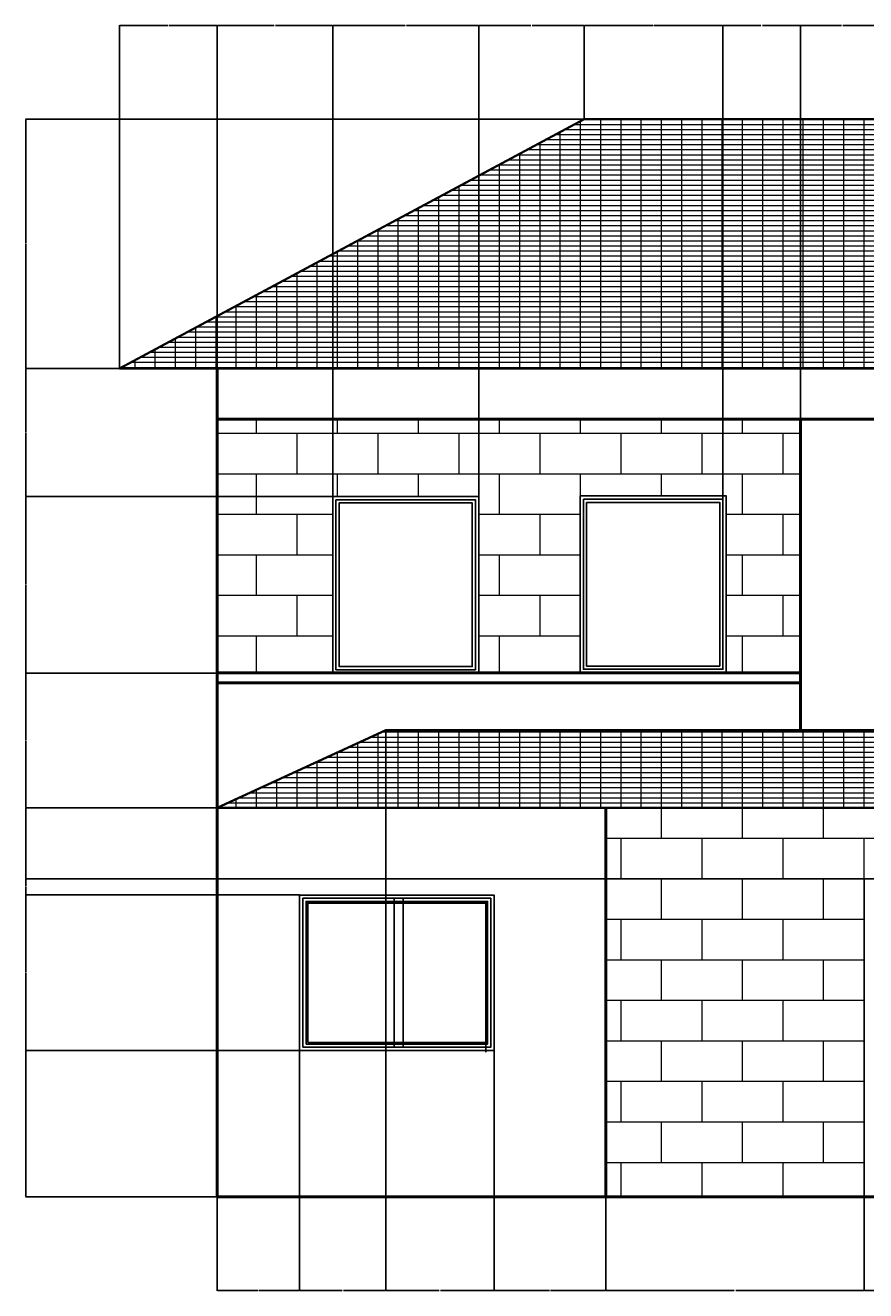
# Model space of a CAD drawing. Units: inches. Extents: x 357 to 1610, y 271 to 1052.
# Tile 1 of 2: x 357 to 876, y 271 to 1052. Entities that reach past the tile are written whole.
import ezdxf

# ---------------------------------------------------------------- set-up
doc = ezdxf.new("R2010")
doc.units = ezdxf.units.IN
doc.header["$MEASUREMENT"] = 0
for name, color, linetype, lineweight in [('A-ANNO-DIMS', 2, 'Continuous', 18), ('A-DOOR', 40, 'Continuous', 25), ('A-GLAZ', 4, 'Continuous', 25), ('A-ROOF', 7, 'Continuous', 35), ('A-ROOF-PATT', 8, 'Continuous', 13), ('A-WALL', 7, 'Continuous', 50), ('A-WALL-PATT', 8, 'Continuous', 18)]:
    doc.layers.add(name, color=color, linetype=linetype, lineweight=lineweight)
doc.styles.get("Standard").update_dxf_attribs({"font": 'arial.ttf'})
doc.dimstyles.get("Standard").update_dxf_attribs({"dimtxt": 0.18, "dimasz": 0.18, "dimexe": 0.18, "dimexo": 0.0625, "dimgap": 0.09, "dimtad": 0, "dimtih": 1, "dimtoh": 1, "dimdec": 4, "dimzin": 0, "dimdsep": 46, "dimtxsty": 'Standard', "dimcen": 0.09, "dimadec": 0, "dimazin": 0, "dimtfac": 1, "dimtdec": 4, "dimtofl": 0, "dimtmove": 0, "dimatfit": 3, "dimfxl": 1, "dimtolj": 1, "dimtzin": 0, "dimarcsym": 0})

# ---------------------------------------------------------------- blocks, each defined once
blk = doc.blocks.new('WIN-900x1090')
for points in [[(0, 108.96), (90.12, 108.96), (90.12, 0), (0, 0)], [(2, 106.96), (88.12, 106.96), (88.12, 2), (2, 2)], [(4, 104.96), (86.12, 104.96), (86.12, 4), (4, 4)]]:
    blk.add_lwpolyline(points, close=True)
blk = doc.blocks.new('*D4')
at = {"layer": 'A-ANNO-DIMS', "color": 0, "lineweight": -2, "transparency": 16777216}
for p, q in [((415.45, 839.95), (415.45, 1051.75)), ((415.63, 1051.57), (445.17, 1051.57)), ((475.49, 1051.57), (445.95, 1051.57)), ((475.67, 839.95), (475.67, 1051.75))]:
    blk.add_line(p, q, dxfattribs=at)
at = {"layer": 'A-ANNO-DIMS', "color": 0, "transparency": 16777216}
for points in [[(415.63, 1051.6), (415.63, 1051.54), (415.45, 1051.57)], [(475.49, 1051.6), (475.49, 1051.54), (475.67, 1051.57)]]:
    blk.add_solid(points, dxfattribs=at)
at = {"layer": 'Defpoints', "color": 0, "transparency": 16777216}
for p in [(475.67, 1051.57), (415.45, 839.89), (475.67, 839.89)]:
    blk.add_point(p, dxfattribs=at)
at = {"layer": 'A-ANNO-DIMS', "color": 0, "transparency": 16777216, "insert": (445.56, 1051.57), "char_height": 0.18, "attachment_point": 5}
blk.add_mtext('\\A1;60.22', dxfattribs=at)
blk = doc.blocks.new('*D5')
at = {"layer": 'A-ANNO-DIMS', "color": 0, "lineweight": -2, "transparency": 16777216}
for p, q in [((475.67, 839.95), (475.67, 1051.75)), ((475.85, 1051.57), (510.96, 1051.57)), ((546.85, 1051.57), (511.74, 1051.57)), ((547.03, 761.02), (547.03, 1051.75))]:
    blk.add_line(p, q, dxfattribs=at)
at = {"layer": 'A-ANNO-DIMS', "color": 0, "transparency": 16777216}
for points in [[(475.85, 1051.6), (475.85, 1051.54), (475.67, 1051.57)], [(546.85, 1051.6), (546.85, 1051.54), (547.03, 1051.57)]]:
    blk.add_solid(points, dxfattribs=at)
at = {"layer": 'Defpoints', "color": 0, "transparency": 16777216}
for p in [(547.03, 1051.57), (475.67, 839.89), (547.03, 760.96)]:
    blk.add_point(p, dxfattribs=at)
at = {"layer": 'A-ANNO-DIMS', "color": 0, "transparency": 16777216, "insert": (511.35, 1051.57), "char_height": 0.18, "attachment_point": 5}
blk.add_mtext('\\A1;71.36', dxfattribs=at)
blk = doc.blocks.new('*D6')
at = {"layer": 'A-ANNO-DIMS', "color": 0, "lineweight": -2, "transparency": 16777216}
for p, q in [((547.03, 761.02), (547.03, 1051.75)), ((547.21, 1051.57), (591.7, 1051.57)), ((636.97, 1051.57), (592.49, 1051.57)), ((637.15, 761.02), (637.15, 1051.75))]:
    blk.add_line(p, q, dxfattribs=at)
at = {"layer": 'A-ANNO-DIMS', "color": 0, "transparency": 16777216}
for points in [[(547.21, 1051.6), (547.21, 1051.54), (547.03, 1051.57)], [(636.97, 1051.6), (636.97, 1051.54), (637.15, 1051.57)]]:
    blk.add_solid(points, dxfattribs=at)
at = {"layer": 'Defpoints', "color": 0, "transparency": 16777216}
for p in [(637.15, 1051.57), (547.03, 760.96), (637.15, 760.96)]:
    blk.add_point(p, dxfattribs=at)
at = {"layer": 'A-ANNO-DIMS', "color": 0, "transparency": 16777216, "insert": (592.09, 1051.57), "char_height": 0.18, "attachment_point": 5}
blk.add_mtext('\\A1;90.12', dxfattribs=at)
blk = doc.blocks.new('*D7')
at = {"layer": 'A-ANNO-DIMS', "color": 0, "lineweight": -2, "transparency": 16777216}
for p, q in [((637.15, 761.02), (637.15, 1051.75)), ((637.33, 1051.57), (669.33, 1051.57)), ((702.11, 1051.57), (670.12, 1051.57)), ((702.29, 993.83), (702.29, 1051.75))]:
    blk.add_line(p, q, dxfattribs=at)
at = {"layer": 'A-ANNO-DIMS', "color": 0, "transparency": 16777216}
for points in [[(637.33, 1051.6), (637.33, 1051.54), (637.15, 1051.57)], [(702.11, 1051.6), (702.11, 1051.54), (702.29, 1051.57)]]:
    blk.add_solid(points, dxfattribs=at)
at = {"layer": 'Defpoints', "color": 0, "transparency": 16777216}
for p in [(702.29, 1051.57), (702.29, 993.77), (637.15, 760.96)]:
    blk.add_point(p, dxfattribs=at)
at = {"layer": 'A-ANNO-DIMS', "color": 0, "transparency": 16777216, "insert": (669.72, 1051.57), "char_height": 0.18, "attachment_point": 5}
blk.add_mtext('\\A1;65.14', dxfattribs=at)
blk = doc.blocks.new('*D8')
at = {"layer": 'A-ANNO-DIMS', "color": 0, "lineweight": -2, "transparency": 16777216}
for p, q in [((702.29, 993.83), (702.29, 1051.75)), ((702.47, 1051.57), (744.76, 1051.57)), ((787.7, 1051.57), (745.41, 1051.57)), ((787.88, 759.31), (787.88, 1051.75))]:
    blk.add_line(p, q, dxfattribs=at)
at = {"layer": 'A-ANNO-DIMS', "color": 0, "transparency": 16777216}
for points in [[(702.47, 1051.6), (702.47, 1051.54), (702.29, 1051.57)], [(787.7, 1051.6), (787.7, 1051.54), (787.88, 1051.57)]]:
    blk.add_solid(points, dxfattribs=at)
at = {"layer": 'Defpoints', "color": 0, "transparency": 16777216}
for p in [(787.88, 1051.57), (702.29, 993.77), (787.88, 759.25)]:
    blk.add_point(p, dxfattribs=at)
at = {"layer": 'A-ANNO-DIMS', "color": 0, "transparency": 16777216, "insert": (745.09, 1051.57), "char_height": 0.18, "attachment_point": 5}
blk.add_mtext('\\A1;85.6', dxfattribs=at)
blk = doc.blocks.new('*D9')
at = {"layer": 'A-ANNO-DIMS', "color": 0, "lineweight": -2, "transparency": 16777216}
for p, q in [((787.88, 759.31), (787.88, 1051.75)), ((788.06, 1051.57), (811.31, 1051.57)), ((835.49, 1051.57), (812.25, 1051.57)), ((835.67, 808.83), (835.67, 1051.75))]:
    blk.add_line(p, q, dxfattribs=at)
at = {"layer": 'A-ANNO-DIMS', "color": 0, "transparency": 16777216}
for points in [[(788.06, 1051.6), (788.06, 1051.54), (787.88, 1051.57)], [(835.49, 1051.6), (835.49, 1051.54), (835.67, 1051.57)]]:
    blk.add_solid(points, dxfattribs=at)
at = {"layer": 'Defpoints', "color": 0, "transparency": 16777216}
for p in [(835.67, 1051.57), (835.67, 808.77), (787.88, 759.25)]:
    blk.add_point(p, dxfattribs=at)
at = {"layer": 'A-ANNO-DIMS', "color": 0, "transparency": 16777216, "insert": (811.78, 1051.57), "char_height": 0.18, "attachment_point": 5}
blk.add_mtext('\\A1;47.785', dxfattribs=at)
blk = doc.blocks.new('*D10')
at = {"layer": 'A-ANNO-DIMS', "color": 0, "lineweight": -2, "transparency": 16777216}
for p, q in [((835.67, 808.83), (835.67, 1051.75)), ((835.85, 1051.57), (861.05, 1051.57)), ((887.04, 1051.57), (861.84, 1051.57)), ((887.22, 769.8), (887.22, 1051.75))]:
    blk.add_line(p, q, dxfattribs=at)
at = {"layer": 'A-ANNO-DIMS', "color": 0, "transparency": 16777216}
for points in [[(835.85, 1051.6), (835.85, 1051.54), (835.67, 1051.57)], [(887.04, 1051.6), (887.04, 1051.54), (887.22, 1051.57)]]:
    blk.add_solid(points, dxfattribs=at)
at = {"layer": 'Defpoints', "color": 0, "transparency": 16777216}
for p in [(887.22, 1051.57), (835.67, 808.77), (887.22, 769.73)]:
    blk.add_point(p, dxfattribs=at)
at = {"layer": 'A-ANNO-DIMS', "color": 0, "transparency": 16777216, "insert": (861.44, 1051.57), "char_height": 0.18, "attachment_point": 5}
blk.add_mtext('\\A1;51.55', dxfattribs=at)
blk = doc.blocks.new('*D22')
at = {"layer": 'A-ANNO-DIMS', "color": 0, "lineweight": -2, "transparency": 16777216}
for p, q in [((526.59, 418.93), (526.59, 270.79)), ((475.67, 328.7), (475.67, 270.79)), ((475.85, 270.97), (500.74, 270.97)), ((526.41, 270.97), (501.52, 270.97))]:
    blk.add_line(p, q, dxfattribs=at)
at = {"layer": 'A-ANNO-DIMS', "color": 0, "transparency": 16777216}
for points in [[(475.85, 271), (475.85, 270.94), (475.67, 270.97)], [(526.41, 271), (526.41, 270.94), (526.59, 270.97)]]:
    blk.add_solid(points, dxfattribs=at)
at = {"layer": 'Defpoints', "color": 0, "transparency": 16777216}
for p in [(526.59, 419), (475.67, 328.77), (526.59, 270.97)]:
    blk.add_point(p, dxfattribs=at)
at = {"layer": 'A-ANNO-DIMS', "color": 0, "transparency": 16777216, "insert": (501.13, 270.97), "char_height": 0.18, "attachment_point": 5}
blk.add_mtext('\\A1;50.92', dxfattribs=at)
blk = doc.blocks.new('*D23')
at = {"layer": 'A-ANNO-DIMS', "color": 0, "lineweight": -2, "transparency": 16777216}
for p, q in [((579.84, 616.7), (579.84, 270.79)), ((526.59, 418.93), (526.59, 270.79)), ((526.77, 270.97), (552.82, 270.97)), ((579.66, 270.97), (553.61, 270.97))]:
    blk.add_line(p, q, dxfattribs=at)
at = {"layer": 'A-ANNO-DIMS', "color": 0, "transparency": 16777216}
for points in [[(526.77, 271), (526.77, 270.94), (526.59, 270.97)], [(579.66, 271), (579.66, 270.94), (579.84, 270.97)]]:
    blk.add_solid(points, dxfattribs=at)
at = {"layer": 'Defpoints', "color": 0, "transparency": 16777216}
for p in [(579.84, 616.77), (526.59, 419), (579.84, 270.97)]:
    blk.add_point(p, dxfattribs=at)
at = {"layer": 'A-ANNO-DIMS', "color": 0, "transparency": 16777216, "insert": (553.22, 270.97), "char_height": 0.18, "attachment_point": 5}
blk.add_mtext('\\A1;53.25', dxfattribs=at)
blk = doc.blocks.new('*D24')
at = {"layer": 'A-ANNO-DIMS', "color": 0, "lineweight": -2, "transparency": 16777216}
for p, q in [((579.84, 616.7), (579.84, 270.79)), ((646.59, 418.93), (646.59, 270.79)), ((580.02, 270.97), (612.82, 270.97)), ((646.41, 270.97), (613.61, 270.97))]:
    blk.add_line(p, q, dxfattribs=at)
at = {"layer": 'A-ANNO-DIMS', "color": 0, "transparency": 16777216}
for points in [[(580.02, 271), (580.02, 270.94), (579.84, 270.97)], [(646.41, 271), (646.41, 270.94), (646.59, 270.97)]]:
    blk.add_solid(points, dxfattribs=at)
at = {"layer": 'Defpoints', "color": 0, "transparency": 16777216}
for p in [(579.84, 616.77), (646.59, 419), (646.59, 270.97)]:
    blk.add_point(p, dxfattribs=at)
at = {"layer": 'A-ANNO-DIMS', "color": 0, "transparency": 16777216, "insert": (613.22, 270.97), "char_height": 0.18, "attachment_point": 5}
blk.add_mtext('\\A1;66.75', dxfattribs=at)
blk = doc.blocks.new('*D25')
at = {"layer": 'A-ANNO-DIMS', "color": 0, "lineweight": -2, "transparency": 16777216}
for p, q in [((646.59, 418.93), (646.59, 270.79)), ((715.67, 328.7), (715.67, 270.79)), ((646.77, 270.97), (680.74, 270.97)), ((715.49, 270.97), (681.53, 270.97))]:
    blk.add_line(p, q, dxfattribs=at)
at = {"layer": 'A-ANNO-DIMS', "color": 0, "transparency": 16777216}
for points in [[(646.77, 271), (646.77, 270.94), (646.59, 270.97)], [(715.49, 271), (715.49, 270.94), (715.67, 270.97)]]:
    blk.add_solid(points, dxfattribs=at)
at = {"layer": 'Defpoints', "color": 0, "transparency": 16777216}
for p in [(646.59, 419), (715.67, 328.77), (715.67, 270.97)]:
    blk.add_point(p, dxfattribs=at)
at = {"layer": 'A-ANNO-DIMS', "color": 0, "transparency": 16777216, "insert": (681.13, 270.97), "char_height": 0.18, "attachment_point": 5}
blk.add_mtext('\\A1;69.08', dxfattribs=at)
blk = doc.blocks.new('*D26')
at = {"layer": 'A-ANNO-DIMS', "color": 0, "lineweight": -2, "transparency": 16777216}
for p, q in [((715.67, 328.7), (715.67, 270.79)), ((875, 328.7), (875, 270.79)), ((715.85, 270.97), (794.88, 270.97)), ((874.82, 270.97), (795.79, 270.97))]:
    blk.add_line(p, q, dxfattribs=at)
at = {"layer": 'A-ANNO-DIMS', "color": 0, "transparency": 16777216}
for points in [[(715.85, 271), (715.85, 270.94), (715.67, 270.97)], [(874.82, 271), (874.82, 270.94), (875, 270.97)]]:
    blk.add_solid(points, dxfattribs=at)
at = {"layer": 'Defpoints', "color": 0, "transparency": 16777216}
for p in [(715.67, 328.77), (875, 328.77), (875, 270.97)]:
    blk.add_point(p, dxfattribs=at)
at = {"layer": 'A-ANNO-DIMS', "color": 0, "transparency": 16777216, "insert": (795.33, 270.97), "char_height": 0.18, "attachment_point": 5}
blk.add_mtext('\\A1;159.33', dxfattribs=at)
blk = doc.blocks.new('*D27')
at = {"layer": 'A-ANNO-DIMS', "color": 0, "lineweight": -2, "transparency": 16777216}
for p, q in [((875, 328.7), (875, 270.79)), ((975, 328.7), (975, 270.79)), ((875.18, 270.97), (924.72, 270.97)), ((974.82, 270.97), (925.28, 270.97))]:
    blk.add_line(p, q, dxfattribs=at)
at = {"layer": 'A-ANNO-DIMS', "color": 0, "transparency": 16777216}
for points in [[(875.18, 271), (875.18, 270.94), (875, 270.97)], [(974.82, 271), (974.82, 270.94), (975, 270.97)]]:
    blk.add_solid(points, dxfattribs=at)
at = {"layer": 'Defpoints', "color": 0, "transparency": 16777216}
for p in [(875, 328.77), (975, 328.77), (975, 270.97)]:
    blk.add_point(p, dxfattribs=at)
at = {"layer": 'A-ANNO-DIMS', "color": 0, "transparency": 16777216, "insert": (925, 270.97), "char_height": 0.18, "attachment_point": 5}
blk.add_mtext('\\A1;100', dxfattribs=at)
blk = doc.blocks.new('*D32')
at = {"layer": 'A-ANNO-DIMS', "color": 0, "lineweight": -2, "transparency": 16777216}
for p, q in [((526.53, 419), (357.47, 419)), ((357.65, 418.82), (357.65, 374.06)), ((357.65, 328.95), (357.65, 373.7)), ((475.61, 328.77), (357.47, 328.77))]:
    blk.add_line(p, q, dxfattribs=at)
at = {"layer": 'A-ANNO-DIMS', "color": 0, "transparency": 16777216}
for points in [[(357.62, 418.82), (357.68, 418.82), (357.65, 419)], [(357.62, 328.95), (357.68, 328.95), (357.65, 328.77)]]:
    blk.add_solid(points, dxfattribs=at)
at = {"layer": 'Defpoints', "color": 0, "transparency": 16777216}
for p in [(357.65, 419), (526.59, 419), (475.67, 328.77)]:
    blk.add_point(p, dxfattribs=at)
at = {"layer": 'A-ANNO-DIMS', "color": 0, "transparency": 16777216, "insert": (357.65, 373.88), "char_height": 0.18, "attachment_point": 5}
blk.add_mtext('\\A1;90.23', dxfattribs=at)
blk = doc.blocks.new('*D33')
at = {"layer": 'A-ANNO-DIMS', "color": 0, "lineweight": -2, "transparency": 16777216}
for p, q in [((526.53, 515), (357.47, 515)), ((357.65, 514.82), (357.65, 467.18)), ((357.65, 419.18), (357.65, 466.81)), ((526.53, 419), (357.47, 419))]:
    blk.add_line(p, q, dxfattribs=at)
at = {"layer": 'A-ANNO-DIMS', "color": 0, "transparency": 16777216}
for points in [[(357.62, 514.82), (357.68, 514.82), (357.65, 515)], [(357.62, 419.18), (357.68, 419.18), (357.65, 419)]]:
    blk.add_solid(points, dxfattribs=at)
at = {"layer": 'Defpoints', "color": 0, "transparency": 16777216}
for p in [(357.65, 515), (526.59, 515), (526.59, 419)]:
    blk.add_point(p, dxfattribs=at)
at = {"layer": 'A-ANNO-DIMS', "color": 0, "transparency": 16777216, "insert": (357.65, 467), "char_height": 0.18, "attachment_point": 5}
blk.add_mtext('\\A1;96', dxfattribs=at)
blk = doc.blocks.new('*D34')
at = {"layer": 'A-ANNO-DIMS', "color": 0, "lineweight": -2, "transparency": 16777216}
for p, q in [((874.94, 525), (357.47, 525)), ((357.65, 524.82), (357.65, 520.18)), ((357.65, 515.18), (357.65, 519.82)), ((526.53, 515), (357.47, 515))]:
    blk.add_line(p, q, dxfattribs=at)
at = {"layer": 'A-ANNO-DIMS', "color": 0, "transparency": 16777216}
for points in [[(357.62, 524.82), (357.68, 524.82), (357.65, 525)], [(357.62, 515.18), (357.68, 515.18), (357.65, 515)]]:
    blk.add_solid(points, dxfattribs=at)
at = {"layer": 'Defpoints', "color": 0, "transparency": 16777216}
for p in [(357.65, 525), (875, 525), (526.59, 515)]:
    blk.add_point(p, dxfattribs=at)
at = {"layer": 'A-ANNO-DIMS', "color": 0, "transparency": 16777216, "insert": (357.65, 520), "char_height": 0.18, "attachment_point": 5}
blk.add_mtext('\\A1;10.004', dxfattribs=at)
blk = doc.blocks.new('*D35')
at = {"layer": 'A-ANNO-DIMS', "color": 0, "lineweight": -2, "transparency": 16777216}
for p, q in [((475.61, 568.77), (357.47, 568.77)), ((357.65, 568.59), (357.65, 547.07)), ((357.65, 525.18), (357.65, 546.7)), ((874.94, 525), (357.47, 525))]:
    blk.add_line(p, q, dxfattribs=at)
at = {"layer": 'A-ANNO-DIMS', "color": 0, "transparency": 16777216}
for points in [[(357.62, 568.59), (357.68, 568.59), (357.65, 568.77)], [(357.62, 525.18), (357.68, 525.18), (357.65, 525)]]:
    blk.add_solid(points, dxfattribs=at)
at = {"layer": 'Defpoints', "color": 0, "transparency": 16777216}
for p in [(357.65, 568.77), (475.67, 568.77), (875, 525)]:
    blk.add_point(p, dxfattribs=at)
at = {"layer": 'A-ANNO-DIMS', "color": 0, "transparency": 16777216, "insert": (357.65, 546.88), "char_height": 0.18, "attachment_point": 5}
blk.add_mtext('\\A1;43.77', dxfattribs=at)
blk = doc.blocks.new('*D36')
at = {"layer": 'A-ANNO-DIMS', "color": 0, "lineweight": -2, "transparency": 16777216}
for p, q in [((546.97, 652), (357.47, 652)), ((357.65, 651.82), (357.65, 610.56)), ((357.65, 568.95), (357.65, 610.2)), ((475.61, 568.77), (357.47, 568.77))]:
    blk.add_line(p, q, dxfattribs=at)
at = {"layer": 'A-ANNO-DIMS', "color": 0, "transparency": 16777216}
for points in [[(357.62, 651.82), (357.68, 651.82), (357.65, 652)], [(357.62, 568.95), (357.68, 568.95), (357.65, 568.77)]]:
    blk.add_solid(points, dxfattribs=at)
at = {"layer": 'Defpoints', "color": 0, "transparency": 16777216}
for p in [(357.65, 652), (547.03, 652), (475.67, 568.77)]:
    blk.add_point(p, dxfattribs=at)
at = {"layer": 'A-ANNO-DIMS', "color": 0, "transparency": 16777216, "insert": (357.65, 610.38), "char_height": 0.18, "attachment_point": 5}
blk.add_mtext('\\A1;83.23', dxfattribs=at)
blk = doc.blocks.new('*D37')
at = {"layer": 'A-ANNO-DIMS', "color": 0, "lineweight": -2, "transparency": 16777216}
for p, q in [((546.97, 760.96), (357.47, 760.96)), ((357.65, 760.78), (357.65, 706.66)), ((357.65, 652.18), (357.65, 706.3)), ((546.97, 652), (357.47, 652))]:
    blk.add_line(p, q, dxfattribs=at)
at = {"layer": 'A-ANNO-DIMS', "color": 0, "transparency": 16777216}
for points in [[(357.62, 760.78), (357.68, 760.78), (357.65, 760.96)], [(357.62, 652.18), (357.68, 652.18), (357.65, 652)]]:
    blk.add_solid(points, dxfattribs=at)
at = {"layer": 'Defpoints', "color": 0, "transparency": 16777216}
for p in [(357.65, 760.96), (547.03, 760.96), (547.03, 652)]:
    blk.add_point(p, dxfattribs=at)
at = {"layer": 'A-ANNO-DIMS', "color": 0, "transparency": 16777216, "insert": (357.65, 706.48), "char_height": 0.18, "attachment_point": 5}
blk.add_mtext('\\A1;108.96', dxfattribs=at)
blk = doc.blocks.new('*D38')
at = {"layer": 'A-ANNO-DIMS', "color": 0, "lineweight": -2, "transparency": 16777216}
for p, q in [((415.39, 839.89), (357.47, 839.89)), ((357.65, 839.71), (357.65, 800.61)), ((357.65, 761.14), (357.65, 800.24)), ((546.97, 760.96), (357.47, 760.96))]:
    blk.add_line(p, q, dxfattribs=at)
at = {"layer": 'A-ANNO-DIMS', "color": 0, "transparency": 16777216}
for points in [[(357.62, 839.71), (357.68, 839.71), (357.65, 839.89)], [(357.62, 761.14), (357.68, 761.14), (357.65, 760.96)]]:
    blk.add_solid(points, dxfattribs=at)
at = {"layer": 'Defpoints', "color": 0, "transparency": 16777216}
for p in [(357.65, 839.89), (415.45, 839.89), (547.03, 760.96)]:
    blk.add_point(p, dxfattribs=at)
at = {"layer": 'A-ANNO-DIMS', "color": 0, "transparency": 16777216, "insert": (357.65, 800.42), "char_height": 0.18, "attachment_point": 5}
blk.add_mtext('\\A1;78.93', dxfattribs=at)
blk = doc.blocks.new('*D39')
at = {"layer": 'A-ANNO-DIMS', "color": 0, "lineweight": -2, "transparency": 16777216}
for p, q in [((702.23, 993.77), (357.47, 993.77)), ((357.65, 993.59), (357.65, 917.01)), ((357.65, 840.07), (357.65, 916.65)), ((415.39, 839.89), (357.47, 839.89))]:
    blk.add_line(p, q, dxfattribs=at)
at = {"layer": 'A-ANNO-DIMS', "color": 0, "transparency": 16777216}
for points in [[(357.62, 993.59), (357.68, 993.59), (357.65, 993.77)], [(357.62, 840.07), (357.68, 840.07), (357.65, 839.89)]]:
    blk.add_solid(points, dxfattribs=at)
at = {"layer": 'Defpoints', "color": 0, "transparency": 16777216}
for p in [(357.65, 993.77), (702.29, 993.77), (415.45, 839.89)]:
    blk.add_point(p, dxfattribs=at)
at = {"layer": 'A-ANNO-DIMS', "color": 0, "transparency": 16777216, "insert": (357.65, 916.83), "char_height": 0.18, "attachment_point": 5}
blk.add_mtext('\\A1;153.88', dxfattribs=at)

msp = doc.modelspace()

# ---------------------------------------------------------------- hatches: boundary and pattern name
at = {"layer": 'A-ROOF-PATT'}
h = msp.add_hatch(dxfattribs=at)
h.set_pattern_fill('GRATE', color=256, scale=100)
h.paths.add_polyline_path([(1006.7419, 993.7706), (702.2918, 993.7706), (415.4488, 839.8897), (475.6698, 839.8897), (1435.5868, 839.8897), (1495.8077, 839.8897), (1350.5849, 901.7507), (1169.5186, 901.7507)])
h = msp.add_hatch(dxfattribs=at)
h.set_pattern_fill('GRATE', color=256, scale=100)
h.paths.add_polyline_path([(1435.6698, 616.7674), (579.8425, 616.7674), (475.6698, 568.7674), (1435.6698, 568.7674), (1551.4751, 568.7674)])
at = {"layer": 'A-WALL-PATT'}
h = msp.add_hatch(dxfattribs=at)
h.set_pattern_fill('BRICK', color=256, scale=100)
h.paths.add_polyline_path([(835.6698, 652.0149), (835.6698, 808.7674), (475.6698, 808.7674), (475.6698, 652.0149), (547.031, 652.0149), (547.031, 760.9583), (637.1546, 760.9583), (637.1546, 652.0149)])
h.paths.add_polyline_path([(699.7613, 761.2521), (789.8849, 761.2521), (789.8849, 652.2919), (699.7613, 652.2919)], flags=16)
h.paths.add_polyline_path([(701.7613, 759.2521), (787.8849, 759.2521), (787.8849, 654.2919), (701.7613, 654.2919)], flags=0)
h.paths.add_polyline_path([(703.7613, 757.2521), (785.8849, 757.2521), (785.8849, 656.2919), (703.7613, 656.2919)], flags=0)
h.paths.add_polyline_path([(1308.107, 761.0593), (1398.2306, 761.0593), (1398.2306, 652.0149), (1435.6698, 652.0149), (1435.6698, 808.7674), (1075.6698, 808.7674), (1075.6698, 652.0149), (1088.1132, 652.0149), (1088.1132, 761.152), (1178.2368, 761.152), (1178.2368, 652.0149), (1308.107, 652.0149)])

# ---------------------------------------------------------------- linework, layer by layer
at = {"layer": 'A-DOOR'}
msp.add_lwpolyline([(975, 525), (975.0913, 525), (975, 328.7674), (875, 328.7674), (875, 525)], close=True, dxfattribs=at)
at = {"layer": 'A-GLAZ'}
for p, q in [((584.9121, 420.9965), (584.9121, 512.9965)), ((590.4612, 420.9965), (590.4612, 512.9965)), ((641.592, 417.9965), (641.592, 509.9965))]:
    msp.add_line(p, q, dxfattribs=at)
for points in [[(526.592, 418.9965), (646.592, 418.9965), (646.592, 514.9965), (526.592, 514.9965)], [(528.592, 420.9965), (644.592, 420.9965), (644.592, 512.9965), (528.592, 512.9965)], [(530.592, 422.9965), (642.592, 422.9965), (642.592, 510.9965), (530.592, 510.9965)], [(531.592, 423.9965), (641.592, 423.9965), (641.592, 509.9965), (531.592, 509.9965)]]:
    msp.add_lwpolyline(points, close=True, dxfattribs=at)
at = {"layer": 'A-ROOF'}
for points in [[(1435.5868, 839.8897), (475.6698, 839.8897), (415.4488, 839.8897), (702.2918, 993.7706), (1006.7419, 993.7706), (1169.5186, 901.7507), (1350.5849, 901.7507), (1495.8077, 839.8897)], [(1435.6698, 568.7674), (475.6698, 568.7674), (579.8425, 616.7674), (1435.6698, 616.7674), (1551.4751, 568.7674)]]:
    msp.add_lwpolyline(points, close=True, dxfattribs=at)
at = {"layer": 'A-WALL'}
for p, q in [((475.6698, 808.7674), (475.6698, 839.8897)), ((475.6698, 808.7674), (1435.6698, 808.7674)), ((475.6698, 328.7674), (475.6698, 808.7674)), ((835.6698, 616.7674), (835.6698, 808.7674)), ((475.6698, 652.0149), (835.6698, 652.0149)), ((475.6698, 646.0149), (835.6698, 646.0149)), ((715.6698, 328.7674), (715.6698, 568.7674)), ((1435.6698, 328.7674), (475.6698, 328.7674))]:
    msp.add_line(p, q, dxfattribs=at)
at = {"layer": 'A-WALL-PATT'}
for p, q in [((750, 550), (750, 568.7674)), ((800, 550), (800, 568.7674)), ((850, 550), (850, 568.7674)), ((715.6698, 550), (1015.6698, 550)), ((725, 525), (725, 550)), ((775, 525), (775, 550)), ((825, 525), (825, 550)), ((875, 525), (875, 550)), ((715.6698, 525), (875, 525)), ((750, 500), (750, 525)), ((800, 500), (800, 525)), ((850, 500), (850, 525)), ((715.6698, 500), (875, 500)), ((725, 475), (725, 500)), ((775, 475), (775, 500)), ((825, 475), (825, 500)), ((875, 475), (875, 500)), ((715.6698, 475), (875, 475)), ((750, 450), (750, 475)), ((800, 450), (800, 475)), ((850, 450), (850, 475)), ((715.6698, 450), (875, 450)), ((725, 425), (725, 450)), ((775, 425), (775, 450)), ((825, 425), (825, 450)), ((875, 425), (875, 450)), ((715.6698, 425), (875, 425)), ((750, 400), (750, 425)), ((800, 400), (800, 425)), ((850, 400), (850, 425)), ((715.6698, 400), (875, 400)), ((725, 375), (725, 400)), ((775, 375), (775, 400)), ((825, 375), (825, 400)), ((875, 375), (875, 400)), ((715.6698, 375), (875, 375)), ((750, 350), (750, 375)), ((800, 350), (800, 375)), ((850, 350), (850, 375)), ((715.6698, 350), (875, 350)), ((725, 328.7674), (725, 350)), ((775, 328.7674), (775, 350)), ((825, 328.7674), (825, 350)), ((875, 328.7674), (875, 350))]:
    msp.add_line(p, q, dxfattribs=at)

# ---------------------------------------------------------------- block references
at = {"layer": 'A-GLAZ'}
for p in [(547.0311, 651.9978), (699.7614, 652.2916)]:
    msp.add_blockref('WIN-900x1090', p, dxfattribs=at)

# ---------------------------------------------------------------- dimensions: what is measured, and where the dimension line sits
at = {"layer": 'A-ANNO-DIMS'}
for base, p1, p2, override, picture, middle in [((475.6698, 1051.5706), (415.4488, 839.8897), (475.6698, 839.8897), {"dimdec": 2, "dimlfac": 1, "dimrnd": 0, "dimzin": 0, "dimdsep": 46, "dimlunit": 2}, '*D4', (445.5593, 1051.5706)), ((547.031, 1051.5706), (475.6698, 839.8897), (547.031, 760.9583), {"dimdec": 2, "dimlfac": 1, "dimrnd": 0, "dimzin": 0, "dimdsep": 46, "dimlunit": 2}, '*D5', (511.3504, 1051.5706)), ((637.1546, 1051.5706), (547.031, 760.9583), (637.1546, 760.9583), {"dimdec": 2, "dimlfac": 1, "dimrnd": 0, "dimzin": 0, "dimdsep": 46, "dimlunit": 2}, '*D6', (592.0928, 1051.5706)), ((702.2918, 1051.5706), (637.1546, 760.9583), (702.2918, 993.7706), {"dimdec": 2, "dimlfac": 1, "dimrnd": 0, "dimzin": 0, "dimdsep": 46, "dimlunit": 2}, '*D7', (669.7232, 1051.5706)), ((787.8849, 1051.5706), (702.2918, 993.7706), (787.8849, 759.2521), {"dimdec": 1, "dimlfac": 1, "dimrnd": 0, "dimzin": 0, "dimdsep": 46, "dimlunit": 2}, '*D8', (745.0884, 1051.5706)), ((835.6698, 1051.5706), (787.8849, 759.2521), (835.6698, 808.7674), {"dimdec": 3, "dimlfac": 1, "dimrnd": 0, "dimzin": 0, "dimdsep": 46, "dimlunit": 2}, '*D9', (811.7773, 1051.5706)), ((887.2189, 1051.5706), (835.6698, 808.7674), (887.2189, 769.7345), {"dimdec": 2, "dimlfac": 1, "dimrnd": 0, "dimzin": 0, "dimdsep": 46, "dimlunit": 2}, '*D10', (861.4444, 1051.5706)), ((579.8425, 270.9674), (526.592, 418.9965), (579.8425, 616.7674), {"dimdec": 2, "dimlfac": 1, "dimrnd": 0, "dimzin": 0, "dimdsep": 46, "dimlunit": 2}, '*D23', (553.2172, 270.9674)), ((646.592, 270.9674), (579.8425, 616.7674), (646.592, 418.9965), {"dimdec": 2, "dimlfac": 1, "dimrnd": 0, "dimzin": 0, "dimdsep": 46, "dimlunit": 2}, '*D24', (613.2172, 270.9674)), ((526.592, 270.9674), (475.6698, 328.7674), (526.592, 418.9965), {"dimdec": 2, "dimlfac": 1, "dimrnd": 0, "dimzin": 0, "dimdsep": 46, "dimlunit": 2}, '*D22', (501.1309, 270.9674)), ((715.6698, 270.9674), (646.592, 418.9965), (715.6698, 328.7674), {"dimdec": 2, "dimlfac": 1, "dimrnd": 0, "dimzin": 0, "dimdsep": 46, "dimlunit": 2}, '*D25', (681.1309, 270.9674)), ((875, 270.9674), (715.6698, 328.7674), (875, 328.7674), {"dimdec": 2, "dimlfac": 1, "dimrnd": 0, "dimzin": 0, "dimdsep": 46, "dimlunit": 2}, '*D26', (795.3349, 270.9674)), ((975, 270.9674), (875, 328.7674), (975, 328.7674), {"dimdec": 0, "dimlfac": 1, "dimrnd": 0, "dimzin": 0, "dimdsep": 46, "dimlunit": 2}, '*D27', (925, 270.9674))]:
    dim = msp.add_linear_dim(base=base, p1=p1, p2=p2, dimstyle='Standard', override=override, dxfattribs=at)
    dim.commit()
    dim.dimension.update_dxf_attribs({"geometry": picture, "text_midpoint": middle})
for base, p1, p2, override, picture, middle in [((357.6488, 993.7706), (415.4488, 839.8897), (702.2918, 993.7706), {"dimdec": 2, "dimlfac": 1, "dimrnd": 0, "dimzin": 0, "dimdsep": 46, "dimlunit": 2}, '*D39', (357.6488, 916.8302)), ((357.6488, 839.8897), (547.031, 760.9583), (415.4488, 839.8897), {"dimdec": 2, "dimlfac": 1, "dimrnd": 0, "dimzin": 0, "dimdsep": 46, "dimlunit": 2}, '*D38', (357.6488, 800.424)), ((357.6488, 760.9583), (547.031, 651.998), (547.031, 760.9583), {"dimdec": 2, "dimlfac": 1, "dimrnd": 0, "dimzin": 0, "dimdsep": 46, "dimlunit": 2}, '*D37', (357.6488, 706.4781)), ((357.6488, 651.998), (475.6698, 568.7674), (547.031, 651.998), {"dimdec": 2, "dimlfac": 1, "dimrnd": 0, "dimzin": 0, "dimdsep": 46, "dimlunit": 2}, '*D36', (357.6488, 610.3827)), ((357.6488, 568.7674), (875, 525), (475.6698, 568.7674), {"dimdec": 2, "dimlfac": 1, "dimrnd": 0, "dimzin": 0, "dimdsep": 46, "dimlunit": 2}, '*D35', (357.6488, 546.8837)), ((357.64881, 525), (526.59199, 514.99646), (875, 525), {"dimdec": 3, "dimlfac": 1, "dimrnd": 0, "dimzin": 0, "dimdsep": 46, "dimlunit": 2}, '*D34', (357.64881, 519.99823)), ((357.6488, 514.9965), (526.592, 418.9965), (526.592, 514.9965), {"dimdec": 0, "dimlfac": 1, "dimrnd": 0, "dimzin": 0, "dimdsep": 46, "dimlunit": 2}, '*D33', (357.6488, 466.9965)), ((357.6488, 418.9965), (475.6698, 328.7674), (526.592, 418.9965), {"dimdec": 2, "dimlfac": 1, "dimrnd": 0, "dimzin": 0, "dimdsep": 46, "dimlunit": 2}, '*D32', (357.6488, 373.8819))]:
    dim = msp.add_linear_dim(base=base, p1=p1, p2=p2, angle=90, dimstyle='Standard', override=override, dxfattribs=at)
    dim.commit()
    dim.dimension.update_dxf_attribs({"geometry": picture, "text_midpoint": middle})

doc.saveas('drawing.dxf')
